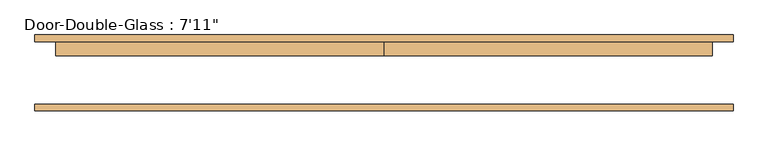
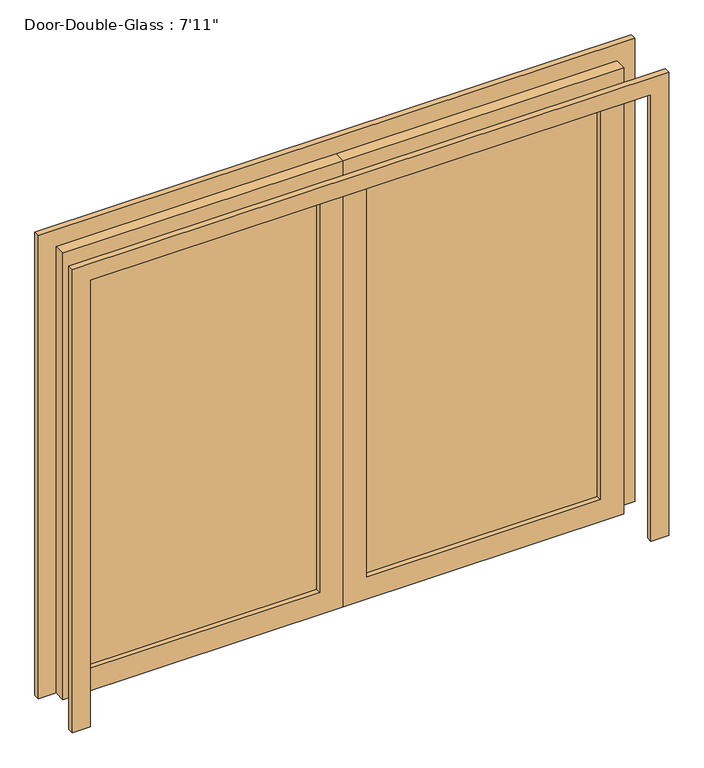
"""IFC4 building model written with IfcOpenShell, lengths in millimetres: door geometry."""

from ifc_helpers import new_model, si_unit, frame, origin, place, context, project, spatial, polyline, outline, extrude, source, transform, mapped, element, save


def door_0e863a58(model_context):
    return source(origin(), model_context, "Body", "SweptSolid", [
        extrude(outline(polyline([(2032.0, 1206.5), (2032.0, 0.0), (0.0, 0.0), (0.0, 1206.5), (2032.0, 1206.5)]), holes=[polyline([(1930.4, 1104.9), (101.6, 1104.9), (101.6, 101.6), (1930.4, 101.6), (1930.4, 1104.9)])]), frame((0.0, 65.88125, 0.0), z_axis=(0.0, 1.0, 0.0), x_axis=(0.0, 0.0, 1.0)), (0.0, 0.0, 1.0), 50.8),
        extrude(outline(polyline([(2032.0, -1206.5), (0.0, -1206.5), (0.0, 0.0), (2032.0, 0.0), (2032.0, -1206.5)]), holes=[polyline([(1930.4, -1104.9), (1930.4, -101.6), (101.6, -101.6), (101.6, -1104.9), (1930.4, -1104.9)])]), frame((0.0, 65.88125, 0.0), z_axis=(0.0, 1.0, 0.0), x_axis=(0.0, 0.0, 1.0)), (0.0, 0.0, 1.0), 50.8),
        extrude(outline(polyline([(-1104.9, 94.45625), (-101.6, 94.45625), (-101.6, 88.10625), (-1104.9, 88.10625), (-1104.9, 94.45625)])), frame((0.0, 0.0, 101.6), z_axis=(0.0, 0.0, 1.0), x_axis=(1.0, 0.0, 0.0)), (0.0, 0.0, 1.0), 1828.8),
        extrude(outline(polyline([(101.6, 94.45625), (1104.9, 94.45625), (1104.9, 88.10625), (101.6, 88.10625), (101.6, 94.45625)])), frame((0.0, 0.0, 101.6), z_axis=(0.0, 0.0, 1.0), x_axis=(1.0, 0.0, 0.0)), (0.0, 0.0, 1.0), 1828.8),
        extrude(outline(polyline([(0.0, 1282.7), (2108.2, 1282.7), (2108.2, -1282.7), (0.0, -1282.7), (0.0, -1206.5), (2032.0, -1206.5), (2032.0, 1206.5), (0.0, 1206.5), (0.0, 1282.7)])), frame((0.0, -137.31875, 0.0), z_axis=(0.0, 1.0, 0.0), x_axis=(0.0, 0.0, 1.0)), (0.0, 0.0, 1.0), 25.4),
        extrude(outline(polyline([(0.0, 1282.7), (2108.2, 1282.7), (2108.2, -1282.7), (0.0, -1282.7), (0.0, -1206.5), (2032.0, -1206.5), (2032.0, 1206.5), (0.0, 1206.5), (0.0, 1282.7)])), frame((0.0, 116.68125, 0.0), z_axis=(0.0, 1.0, 0.0), x_axis=(0.0, 0.0, 1.0)), (0.0, 0.0, 1.0), 25.4),
    ])


if __name__ == "__main__":
    model = new_model("IFC4")
    model_context = context("Model", 3, world=origin())
    ifc_project = project(units=[si_unit("LENGTHUNIT", "METRE", prefix="MILLI")], contexts=[model_context])
    site = spatial("IfcSite", under=ifc_project)
    building = spatial("IfcBuilding", under=site)
    placement = place(None, origin())
    door_shape = door_0e863a58(model_context)
    element("IfcDoor", 1, ObjectType="Door-Double-Glass : 7'11\"", at=placement, inside=building, context=model_context, shape_type="MappedRepresentation", body=[
        mapped(door_shape, transform((0.0, 0.0, 0.0), x_axis=(1.0, 0.0, 0.0), y_axis=(0.0, 1.0, 0.0), z_axis=(0.0, 0.0, 1.0))),
    ])
    save(model, "model.ifc")

# Revit data of these elements
# Type "Door-Double-Glass : 7'11\""
#   Type Mark = "12"
#   Construction Type Id = "opn-d45"
#   Assembly Code = "C1020"
#   Analytic Construction = "Wood frame, double glass door "
#   W = 3' - 11 1/2"
#   Thickness = 0' - 2"
#   Thermal Resistance (R) = 1.8150 (h·ft²·°F)/BTU
#   Swing Angle [instance default] = 90.00°
#   Heat Transfer Coefficient (U) = 0.5510 BTU/(h·ft²·°F)
#   Height = 6' - 8"
#   Bottom Rail = 0' - 4"
#   Top Rail = 0' - 4"
#   Stiles = 0' - 4"
#   Trim Projection = 0' - 1"
#   Trim Width = 0' - 3"
#   Width = 7' - 11"
#   Define Thermal Properties by = 1
#   Glazing = Glass
#   Panel Material = Wood - Birch - Solid Stained Light Low Gloss
#   Trim Material = Paint - Sienna
#   Visual Light Transmittance = 0
#   Solar Heat Gain Coefficient = 0
#   Function = (empty or 0)
#   Wall Closure = (empty or 0)
# Element 1 (IfcDoor, "Door-Double-Glass : 7'11\"")
#   Materials on its faces: "Wood - Birch - Solid Stained Light Low Gloss", "Paint - Sienna", "Glass"
# Materials
#   "Glass": class "Glass", colour RGB 154 182 205, transparency 0.85, Description = "Soda Lime Glass", Cost = 0
#   "Wood - Birch - Solid Stained Light Low Gloss": class "Wood", colour RGB 210 159 95, transparency 0, Cost = 0
#   "Paint - Sienna": colour RGB 118 70 51, transparency 0, Cost = 0
